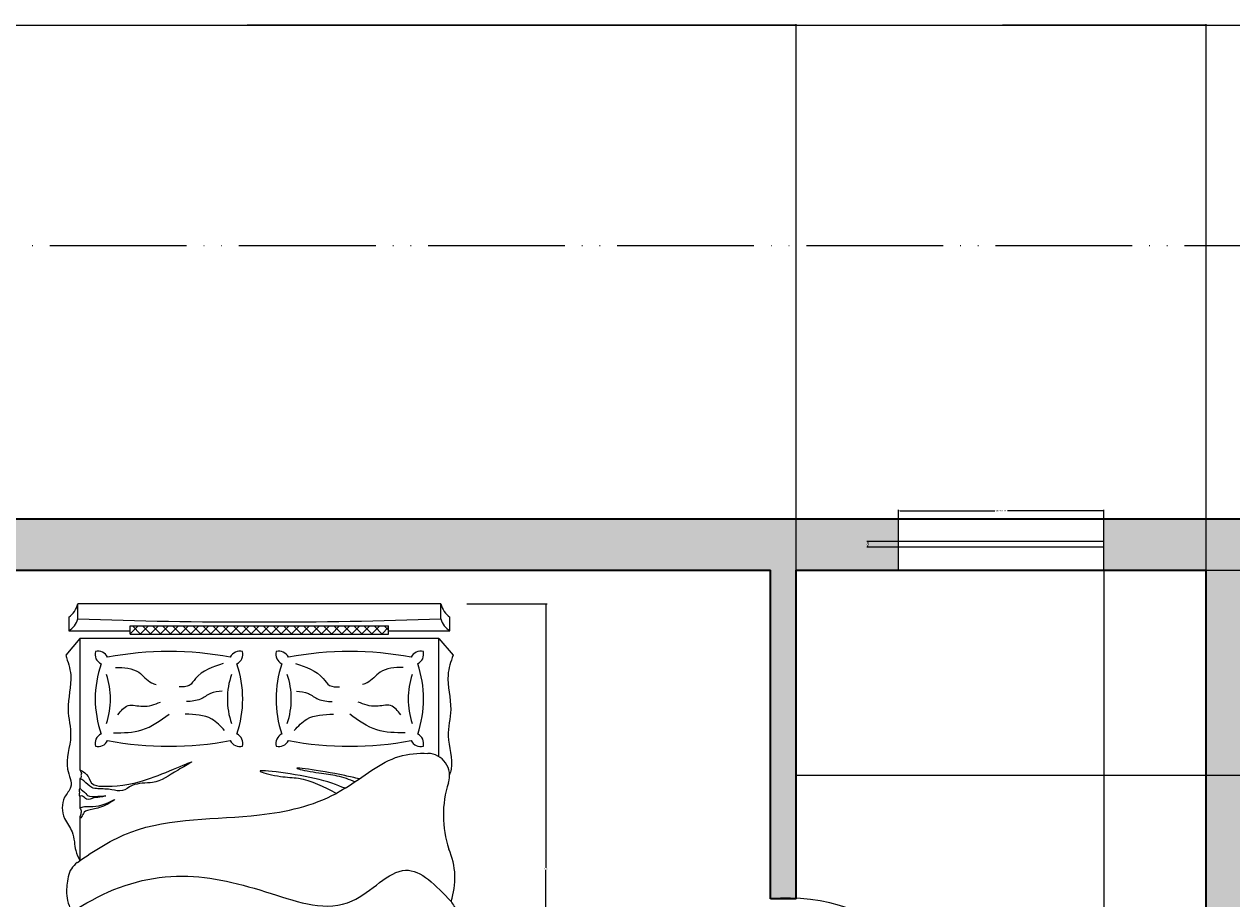
# Model space of a CAD drawing. Units: inches. Extents: x 2847 to 3693, y 1516 to 2098.
# Tile 4 of 6: x 3047 to 3259, y 1944 to 2098. Entities that reach past the tile are written whole.
import ezdxf

# ---------------------------------------------------------------- set-up
doc = ezdxf.new("R2010")
doc.units = ezdxf.units.IN
doc.linetypes.add('ACAD_ISO05W100', pattern=[33, 24, -3, 0, -3, 0, -3])
for name, color, linetype, lineweight in [('A-ANNO-DIMS', 2, 'Continuous', 18), ('A-DOOR', 3, 'Continuous', 18), ('A-FLOR-FIXT', 9, 'Continuous', 18), ('A-FURN', 8, 'Continuous', 18), ('A-GLAZ', 4, 'Continuous', 18), ('A-WALL', 7, 'Continuous', 35), ('C-PROP', 7, 'ACAD_ISO05W100', 18), ('www.cadblocksfree.com', 7, 'Continuous', 9)]:
    doc.layers.add(name, color=color, linetype=linetype, lineweight=lineweight)
doc.layers.add('A-WALL-PATT', color=251, linetype='Continuous', lineweight=13, true_color=0x636466)
doc.styles.get("Standard").update_dxf_attribs({"font": 'arial.ttf'})
doc.dimstyles.get("Standard").update_dxf_attribs({"dimtxt": 0.18, "dimasz": 0.18, "dimexe": 0.18, "dimexo": 0.0625, "dimgap": 0.09, "dimtad": 0, "dimtih": 1, "dimtoh": 1, "dimdec": 4, "dimzin": 0, "dimdsep": 46, "dimtxsty": 'Standard', "dimcen": 0.09, "dimadec": 0, "dimazin": 0, "dimtfac": 1, "dimtdec": 4, "dimtofl": 0, "dimtmove": 0, "dimatfit": 3, "dimfxl": 1, "dimtolj": 1, "dimtzin": 0, "dimarcsym": 0})

# ---------------------------------------------------------------- blocks, each defined once
blk = doc.blocks.new('bed')
at = {"layer": 'www.cadblocksfree.com', "ltscale": 0.2}
h = blk.add_hatch(dxfattribs=at)
h.set_pattern_fill('ANSI37,_O', color=256, scale=0.393701)
h.set_pattern_definition([(45, (2420.7222, -262.9689), (-0.8838835, 0.8838835), []), (135, (2420.7222, -262.9689), (-0.8838835, -0.8838835), [])])
h.paths.add_polyline_path([(3417.57, 1472.4), (3372.19, 1472.4), (3372.19, 1470.94), (3417.57, 1470.94)])
for p, q in [((3363, 1473.59), (3363, 1476.25)), ((3426.76, 1473.59), (3426.76, 1476.25)), ((3372.19, 1472.4), (3417.57, 1472.4)), ((3372.19, 1470.94), (3372.19, 1472.4)), ((3417.57, 1470.94), (3417.57, 1472.4)), ((3363.39, 1470.15), (3360.88, 1467.22)), ((3372.19, 1470.94), (3417.57, 1470.94)), ((3426.38, 1470.15), (3428.88, 1467.22)), ((3409.94, 1443.85), (3408.41, 1442.96)), ((3363.39, 1412.3), (3363.39, 1402.94)), ((3426.38, 1399.91), (3426.38, 1410.81)), ((3363.39, 1391.41), (3426.38, 1391.41))]:
    blk.add_line(p, q, dxfattribs=at)
for points in [[(3426.76, 1476.25), (3363, 1476.25)], [(3361.42, 1473.89), (3361.42, 1471.52), (3372.19, 1471.52)], [(3417.57, 1471.52), (3428.35, 1471.52), (3428.35, 1473.89)], [(3426.38, 1449.41), (3426.38, 1470.15), (3363.39, 1470.15), (3363.39, 1447.08)], [(3363.39, 1445.54), (3363.39, 1443.89)], [(3363.39, 1442.49), (3363.39, 1440.37)], [(3363.39, 1438.56), (3363.39, 1431.14)]]:
    blk.add_lwpolyline(points, dxfattribs=at)
for centre, radius, start, end in [((3359.33, 1477), 3.74, 303.8271, 348.4775), ((3430.43, 1477), 3.74, 191.5225, 236.1729), ((3359.84, 1474.37), 3.25, 298.9176, 345.9939), ((3394.88, 2431.36), 958.3, 268.09356, 271.90644), ((3429.92, 1474.37), 3.25, 194.0061, 241.0824), ((3367.9, 1467.4), 1.87, 165.5166, 244.2099), ((3366.56, 1466.05), 1.87, 25.7901, 104.4834), ((3379.01, 1409.19), 58.68, 79.4235, 100.5765), ((3391.47, 1466.05), 1.87, 75.5166, 154.2099), ((3390.12, 1467.4), 1.87, 295.7901, 14.4834), ((3399.64, 1467.4), 1.87, 165.5166, 244.2099), ((3398.3, 1466.05), 1.87, 25.7901, 104.4834), ((3410.75, 1409.19), 58.68, 79.4235, 100.5765), ((3423.21, 1466.05), 1.87, 75.5166, 154.2099), ((3421.86, 1467.4), 1.87, 295.7901, 14.4834), ((3385.29, 1459.55), 19.22, 161.2852, 198.7148), ((3372.74, 1459.55), 19.22, 341.2852, 18.7148), ((3417.03, 1459.55), 19.22, 161.2852, 198.7148), ((3404.48, 1459.55), 19.22, 341.2852, 18.7148), ((3355.42, 1459.55), 13.34, 341.1598, 18.8402), ((3402.61, 1459.55), 13.34, 161.1598, 198.8402), ((3387.15, 1459.55), 13.34, 341.1598, 18.8402), ((3434.35, 1459.55), 13.34, 161.1598, 198.8402), ((3367.9, 1451.7), 1.87, 115.7901, 194.4834), ((3390.12, 1451.7), 1.87, 345.5166, 64.2099), ((3399.64, 1451.7), 1.87, 115.7901, 194.4834), ((3421.86, 1451.7), 1.87, 345.5166, 64.2099), ((3366.56, 1453.04), 1.87, 255.5166, 334.2099), ((3379.01, 1509.91), 58.68, 259.4235, 280.5765), ((3391.47, 1453.04), 1.87, 205.7901, 284.4834), ((3398.3, 1453.04), 1.87, 255.5166, 334.2099), ((3410.75, 1509.91), 58.68, 259.4235, 280.5765), ((3423.21, 1453.04), 1.87, 205.7901, 284.4834), ((3424.34, 1446.05), 3.94, 342.0511, 87.9851), ((3445.78, 1439.1), 18.6, 162.0511, 198.5657), ((3416.57, 1428.08), 12.65, 341.0268, 23.7782), ((3365.21, 1427.6), 3.94, 125.4209, 169.6982), ((3370.55, 1414.19), 11.47, 139.4648, 203.3712), ((3367.28, 1412.87), 7.94, 204.0179, 212.619), ((3331.91, 1405.56), 34.38, 336.8495, 357.9003), ((3438.82, 1397.31), 13.77, 176.7525, 205.373), ((3432.14, 1393.64), 6.17, 162.6475, 201.1361), ((3422.11, 1384.8), 7.8, 58.0013, 91.6551)]:
    blk.add_arc(centre, radius, start, end, dxfattribs=at)
at = {"layer": 'www.cadblocksfree.com', "ltscale": 0.2, "extrusion": (0, 0, -1)}
for centre, major_axis, ratio, start_param, end_param in [((3360.34, 1388.37), (3.04, 3.04), 0.168252, 4.250342, 8.316029), ((3359.29, 1387.32), (1.05, 1.05), 0.453532, 4.422107, 8.144264)]:
    blk.add_ellipse(centre, major_axis=major_axis, ratio=ratio, start_param=start_param, end_param=end_param, dxfattribs=at)
at = {"layer": 'www.cadblocksfree.com', "ltscale": 0.2}
for centre, major_axis, ratio, start_param, end_param in [((3429.42, 1388.37), (-3.04, 3.04), 0.168252, 4.250342, 8.316029), ((3430.48, 1387.32), (-1.05, 1.05), 0.453532, 4.422107, 8.144264)]:
    blk.add_ellipse(centre, major_axis=major_axis, ratio=ratio, start_param=start_param, end_param=end_param, dxfattribs=at)
for points, knots in [([(3360.88, 1467.22), (3361.27, 1466.08), (3362.33, 1462.98), (3360.73, 1458.15), (3362.39, 1452.62), (3360.35, 1448.14), (3362.43, 1444.24), (3360.04, 1441.93), (3360.26, 1438.68), (3362.05, 1436.55), (3362.42, 1434.52), (3362.57, 1432.76), (3363.1, 1431.71), (3363.39, 1431.14)], [0, 0, 0, 0, 3.550403, 9.643115, 14.356056, 20.206026, 23.427697, 25.46537, 29.172767, 31.884544, 33.668442, 35.237641, 37.145618, 37.145618, 37.145618, 37.145618]), ([(3428.88, 1467.22), (3428.49, 1466.08), (3427.44, 1462.98), (3429.04, 1458.15), (3427.38, 1452.62), (3429.08, 1448.87), (3428.37, 1446.52), (3428.27, 1446.19)], [0, 0, 0, 0, 0.0901802, 0.2449351, 0.3646438, 0.5132331, 0.5378548, 0.5378548, 0.5378548, 0.5378548]), ([(3369.63, 1465.08), (3371.1, 1465.04), (3373.63, 1464.97), (3375.26, 1462.52), (3376.48, 1462.17), (3376.75, 1462.09)], [0, 0, 0, 0, 4.163459, 7.093919, 7.934624, 7.934624, 7.934624, 7.934624]), ([(3388.54, 1465.74), (3386.72, 1465.16), (3384.36, 1464.41), (3382.68, 1461.63), (3381.45, 1461.64), (3380.81, 1461.64)], [0, 0, 0, 0, 5.530688, 7.154877, 8.940839, 8.940839, 8.940839, 8.940839]), ([(3401.22, 1465.74), (3403.05, 1465.16), (3405.41, 1464.41), (3407.09, 1461.63), (3408.31, 1461.64), (3408.95, 1461.64)], [0, 0, 0, 0, 5.530688, 7.154877, 8.940839, 8.940839, 8.940839, 8.940839]), ([(3420.14, 1465.08), (3418.66, 1465.04), (3416.14, 1464.97), (3414.5, 1462.52), (3413.28, 1462.17), (3413.01, 1462.09)], [0, 0, 0, 0, 4.163459, 7.093919, 7.934624, 7.934624, 7.934624, 7.934624]), ([(3388.36, 1460.93), (3387.64, 1460.85), (3386.25, 1460.69), (3384.48, 1459.22), (3382.96, 1459.13), (3382.11, 1459.07)], [0, 0, 0, 0, 2.127543, 4.10272, 6.58647, 6.58647, 6.58647, 6.58647]), ([(3401.41, 1460.93), (3402.13, 1460.85), (3403.51, 1460.69), (3405.28, 1459.22), (3406.81, 1459.13), (3407.65, 1459.07)], [0, 0, 0, 0, 2.127543, 4.10272, 6.58647, 6.58647, 6.58647, 6.58647]), ([(3370.05, 1456.77), (3370.59, 1457.46), (3371.71, 1458.88), (3374.68, 1457.89), (3376.51, 1458.59), (3377.52, 1458.99)], [0, 0, 0, 0, 2.388143, 4.935423, 8.166198, 8.166198, 8.166198, 8.166198]), ([(3419.72, 1456.77), (3419.17, 1457.46), (3418.05, 1458.88), (3415.08, 1457.89), (3413.26, 1458.59), (3412.24, 1458.99)], [0, 0, 0, 0, 2.388143, 4.935423, 8.166198, 8.166198, 8.166198, 8.166198]), ([(3369.29, 1453.58), (3371, 1453.6), (3374.59, 1453.64), (3377.5, 1455.76), (3379.02, 1456.87)], [0, 0, 0, 0, 5.002087, 10.507046, 10.507046, 10.507046, 10.507046]), ([(3388.77, 1454), (3388.07, 1454.76), (3386.27, 1456.73), (3383.54, 1456.81), (3381.88, 1456.86)], [0, 0, 0, 0, 3.013696, 7.735839, 7.735839, 7.735839, 7.735839]), ([(3401, 1454), (3401.7, 1454.76), (3403.5, 1456.73), (3406.22, 1456.81), (3407.88, 1456.86)], [0, 0, 0, 0, 3.013696, 7.735839, 7.735839, 7.735839, 7.735839]), ([(3420.48, 1453.58), (3418.77, 1453.6), (3415.18, 1453.64), (3412.27, 1455.76), (3410.74, 1456.87)], [0, 0, 0, 0, 5.002087, 10.507046, 10.507046, 10.507046, 10.507046]), ([(3367.27, 1444.2), (3369.57, 1444.23), (3373.92, 1444.28), (3385.47, 1449.8), (3379.56, 1446.49), (3376.81, 1444.48), (3372.95, 1444.92), (3370.93, 1443.14), (3368.77, 1443.7), (3367.36, 1443.75), (3366.55, 1443.78)], [0, 0, 0, 0, 8.61026, 16.221274, 18.843057, 23.804898, 27.440828, 29.356102, 31.203478, 33.650687, 33.650687, 33.650687, 33.650687]), ([(3409.94, 1443.85), (3413.12, 1445.84), (3417.43, 1449.66), (3422.72, 1450.04), (3424.48, 1449.98)], [1.3582378, 1.3582378, 1.3582378, 1.3582378, 1.6381418, 1.7706953, 1.7706953, 1.7706953, 1.7706953]), ([(3363.39, 1447.08), (3363.43, 1446.99), (3363.53, 1446.78), (3363.73, 1446.46), (3363.51, 1446.15), (3363.66, 1445.9), (3363.56, 1445.67), (3363.44, 1445.58), (3363.39, 1445.54)], [0, 0, 0, 0, 0.293454, 0.701471, 1.003873, 1.254893, 1.47342, 1.69185, 1.69185, 1.69185, 1.69185]), ([(3363.39, 1447.08), (3363.99, 1446.78), (3365.08, 1446.12), (3365.12, 1444.37), (3367.13, 1444.19), (3367.27, 1444.2)], [0.0122268, 0.0122268, 0.0122268, 0.0122268, 0.0594721, 0.1062177, 0.134458, 0.134458, 0.134458, 0.134458]), ([(3409.94, 1443.85), (3408.47, 1444.45), (3404.44, 1446.04), (3391.4, 1447.6), (3398.64, 1445.77), (3402.97, 1445.76), (3406.22, 1444.09), (3408.41, 1442.96)], [0.0056315, 0.0056315, 0.0056315, 0.0056315, 0.1489731, 0.3882761, 0.4793617, 0.5593494, 0.7397317, 0.7397317, 0.7397317, 0.7397317]), ([(3412.4, 1445.5), (3411.61, 1445.7), (3406.24, 1446.93), (3398.17, 1447.93), (3405.4, 1446.46), (3408.57, 1446.19), (3410.63, 1445.46), (3411.68, 1445)], [0.1043639, 0.1043639, 0.1043639, 0.1043639, 0.1489731, 0.3882761, 0.4793617, 0.5593494, 0.6446217, 0.6446217, 0.6446217, 0.6446217]), ([(3363.39, 1443.89), (3363.33, 1443.81), (3363.17, 1443.56), (3363.35, 1443.12), (3363.23, 1442.79), (3363.23, 1442.53), (3363.34, 1442.51), (3363.39, 1442.49)], [0, 0, 0, 0, 0.27176, 0.887321, 1.189132, 1.388142, 1.515331, 1.515331, 1.515331, 1.515331]), ([(3366.55, 1443.78), (3366.17, 1443.78), (3365.17, 1443.9), (3364.4, 1444.96), (3363.63, 1445.46), (3363.39, 1445.54)], [0.15648839, 0.15648839, 0.15648839, 0.15648839, 0.18439755, 0.23137648, 0.25059846, 0.25059846, 0.25059846, 0.25059846]), ([(3363.39, 1443.89), (3363.63, 1443.61), (3364.67, 1442.73), (3364.89, 1442.15), (3369.07, 1442.74), (3366.77, 1442.24), (3365.83, 1442.3), (3364.61, 1441.55), (3363.96, 1442.54), (3363.54, 1442.52), (3363.39, 1442.49)], [0.0595743, 0.0595743, 0.0595743, 0.0595743, 0.0807529, 0.1037415, 0.1697201, 0.1760361, 0.2071372, 0.2404744, 0.2623409, 0.2736605, 0.2736605, 0.2736605, 0.2736605]), ([(3362.93, 1430.81), (3365.94, 1432.96), (3375.45, 1438.99), (3392.12, 1438.03), (3404.25, 1440.73), (3408.41, 1442.96)], [0.102872, 0.102872, 0.102872, 0.102872, 0.37972, 0.957702, 1.313793, 1.313793, 1.313793, 1.313793]), ([(3363.39, 1440.37), (3363.63, 1440.51), (3364.53, 1440.9), (3366.48, 1440.25), (3370.2, 1442.29), (3367.73, 1440.64), (3365.42, 1440.07), (3364.04, 1439.91), (3363.8, 1438.94), (3363.48, 1438.64), (3363.39, 1438.56)], [0.013856, 0.013856, 0.013856, 0.013856, 0.0348738, 0.0888667, 0.1078792, 0.1267378, 0.158714, 0.1937575, 0.2174868, 0.2267221, 0.2267221, 0.2267221, 0.2267221]), ([(3363.39, 1440.37), (3363.44, 1440.27), (3363.57, 1440.06), (3363.61, 1439.68), (3363.53, 1439.31), (3363.41, 1439), (3363.33, 1438.75), (3363.37, 1438.61), (3363.39, 1438.56)], [0, 0, 0, 0, 0.329977, 0.725302, 1.129072, 1.442831, 1.734218, 1.878348, 1.878348, 1.878348, 1.878348]), ([(3365.51, 1424.21), (3370.52, 1427), (3381.15, 1429.83), (3396.21, 1425.87), (3410.54, 1420.65), (3420.27, 1432.69), (3425.88, 1426.77), (3428.53, 1423.97)], [0.099185, 0.099185, 0.099185, 0.099185, 0.523647, 0.927087, 1.289918, 1.564439, 1.810555, 1.810555, 1.810555, 1.810555]), ([(3361.34, 1428.31), (3361.33, 1428.3), (3361.16, 1427.34), (3360.78, 1425.17), (3361.47, 1423.14), (3362.01, 1421.85)], [0.3128349, 0.3128349, 0.3128349, 0.3128349, 0.313751, 0.386958, 0.4759027, 0.4759027, 0.4759027, 0.4759027]), ([(3428.53, 1423.97), (3428.91, 1423.4), (3430.1, 1421.61), (3428.49, 1417.66), (3430.59, 1413.79), (3429.8, 1409.12), (3428.4, 1406.56), (3427.36, 1404.97)], [0, 0, 0, 0, 0.050513, 0.157399, 0.2842023, 0.3628173, 0.5066917, 0.5066917, 0.5066917, 0.5066917]), ([(3362.06, 1409.87), (3363.64, 1413.65), (3372.98, 1421.34), (3389.68, 1406.04), (3402.4, 1419.98), (3416.04, 1420.17), (3423.23, 1415.23), (3427.83, 1408.9)], [0.029901, 0.029901, 0.029901, 0.029901, 0.276967, 0.797115, 1.093669, 1.464666, 1.788489, 1.788489, 1.788489, 1.788489]), ([(3431.24, 1387.47), (3430.88, 1388.17), (3430.2, 1389.5), (3431.48, 1391.99), (3428.29, 1393.19), (3430.5, 1395.69), (3427.56, 1397.87), (3431.84, 1400.39), (3426.54, 1404.33), (3426.44, 1408.15), (3426.38, 1410.81)], [0, 0, 0, 0, 2.267059, 4.324559, 6.685584, 8.878641, 11.121502, 14.300359, 17.755284, 25.682856, 25.682856, 25.682856, 25.682856]), ([(3358.53, 1387.47), (3359.1, 1389.21), (3359.96, 1391.82), (3361.92, 1395.15), (3361.9, 1398.55), (3359.88, 1401.84), (3361.56, 1405.21), (3361.03, 1407.51), (3360.64, 1408.47), (3360.59, 1408.59)], [0, 0, 0, 0, 0.138875, 0.2092702, 0.2901949, 0.3858479, 0.4804923, 0.5489252, 0.5590752, 0.5590752, 0.5590752, 0.5590752]), ([(3368.63, 1397.84), (3375.98, 1400.49), (3385.35, 1402.76), (3397.53, 1395.27), (3413.59, 1410.38), (3407.81, 1395.02), (3420.76, 1398.2)], [0.029901, 0.029901, 0.029901, 0.029901, 0.276967, 0.797115, 1.093669, 1.16836, 1.16836, 1.16836, 1.16836]), ([(3430.32, 1386.56), (3427.33, 1387.65), (3422.15, 1389.55), (3414.53, 1384.14), (3405.61, 1387.05), (3396.29, 1386.31), (3386.84, 1381.28), (3377.74, 1390.27), (3370.78, 1384.8), (3364.63, 1383.97), (3363.28, 1388.27), (3360.78, 1387.15), (3359.45, 1386.56)], [0, 0, 0, 0, 8.93042, 15.449194, 25.485629, 34.878505, 43.598887, 54.554403, 64.16647, 67.461673, 70.610457, 74.213583, 74.213583, 74.213583, 74.213583])]:
    blk.add_open_spline(points, degree=3, knots=knots, dxfattribs=at)
for points in [[(3361.23, 1424.04), (3361.24, 1424.04), (3361.24, 1424.04), (3361.24, 1424.04)], [(3361.84, 1421.64), (3362.35, 1422.25), (3362.87, 1422.86), (3365.51, 1424.21)]]:
    blk.add_open_spline(points, degree=3, dxfattribs=at)
blk = doc.blocks.new('WIN-GLAZ-36IN')
for p, q in [((36, 1), (0, 1)), ((36, 0), (0, 0))]:
    blk.add_line(p, q)
blk = doc.blocks.new('*D17')
at = {"layer": 'A-ANNO-DIMS', "color": 0, "lineweight": -2, "transparency": 16777216}
for p, q in [((3200.85, 2007.18), (3200.85, 2012.7)), ((3201.03, 2012.52), (3217.73, 2012.52)), ((3236.67, 2012.52), (3219.96, 2012.52)), ((3236.85, 2007.18), (3236.85, 2012.7))]:
    blk.add_line(p, q, dxfattribs=at)
at = {"layer": 'A-ANNO-DIMS', "color": 0, "transparency": 16777216}
for points in [[(3201.03, 2012.55), (3201.03, 2012.49), (3200.85, 2012.52)], [(3236.67, 2012.55), (3236.67, 2012.49), (3236.85, 2012.52)]]:
    blk.add_solid(points, dxfattribs=at)
at = {"layer": 'Defpoints', "color": 0, "transparency": 16777216}
for p in [(3236.85, 2012.52), (3200.85, 2007.12), (3236.85, 2007.12)]:
    blk.add_point(p, dxfattribs=at)
at = {"layer": 'A-ANNO-DIMS', "color": 0, "transparency": 16777216, "insert": (3218.85, 2012.52), "char_height": 0.18, "attachment_point": 5}
blk.add_mtext('\\A1;WINDOW 36 TYP.', dxfattribs=at)
blk = doc.blocks.new('*D18')
at = {"layer": 'A-ANNO-DIMS', "color": 0, "lineweight": -2, "transparency": 16777216}
for p, q in [((3200.78, 2007.12), (3195.27, 2007.12)), ((3200.78, 2006.12), (3195.27, 2006.12)), ((3195.45, 2006.94), (3195.45, 2006.8)), ((3195.45, 2006.3), (3195.45, 2006.44))]:
    blk.add_line(p, q, dxfattribs=at)
at = {"layer": 'A-ANNO-DIMS', "color": 0, "transparency": 16777216}
for points in [[(3195.42, 2006.94), (3195.48, 2006.94), (3195.45, 2007.12)], [(3195.42, 2006.3), (3195.48, 2006.3), (3195.45, 2006.12)]]:
    blk.add_solid(points, dxfattribs=at)
at = {"layer": 'Defpoints', "color": 0, "transparency": 16777216}
for p in [(3195.45, 2007.12), (3200.85, 2007.12), (3200.85, 2006.12)]:
    blk.add_point(p, dxfattribs=at)
at = {"layer": 'A-ANNO-DIMS', "color": 0, "transparency": 16777216, "insert": (3195.45, 2006.62), "char_height": 0.18, "attachment_point": 5}
blk.add_mtext('\\A1;1 TYP.', dxfattribs=at)
blk = doc.blocks.new('*D21')
at = {"layer": 'A-ANNO-DIMS', "color": 0, "lineweight": -2, "transparency": 16777216}
for p, q in [((3125.04, 1996.19), (3139.12, 1996.19)), ((3138.94, 1996.01), (3138.94, 1949.83)), ((3138.94, 1903.3), (3138.94, 1949.47)), ((3125.04, 1903.12), (3139.12, 1903.12))]:
    blk.add_line(p, q, dxfattribs=at)
at = {"layer": 'A-ANNO-DIMS', "color": 0, "transparency": 16777216}
for points in [[(3138.91, 1996.01), (3138.97, 1996.01), (3138.94, 1996.19)], [(3138.91, 1903.3), (3138.97, 1903.3), (3138.94, 1903.12)]]:
    blk.add_solid(points, dxfattribs=at)
at = {"layer": 'Defpoints', "color": 0, "transparency": 16777216}
for p in [(3124.97, 1996.19), (3138.94, 1996.19), (3124.97, 1903.12)]:
    blk.add_point(p, dxfattribs=at)
at = {"layer": 'A-ANNO-DIMS', "color": 0, "transparency": 16777216, "insert": (3138.94, 1949.65), "char_height": 0.18, "attachment_point": 5}
blk.add_mtext('\\A1;BED 93', dxfattribs=at)
blk = doc.blocks.new('*D35')
at = {"layer": 'A-ANNO-DIMS', "color": 0, "lineweight": -2, "transparency": 16777216}
for p, q in [((2885.85, 2059.18), (2885.85, 2098)), ((2886.03, 2097.82), (3269.56, 2097.82)), ((3653.67, 2097.82), (3270.13, 2097.82)), ((3653.85, 2059.18), (3653.85, 2098))]:
    blk.add_line(p, q, dxfattribs=at)
at = {"layer": 'A-ANNO-DIMS', "color": 0, "transparency": 16777216}
for points in [[(2886.03, 2097.85), (2886.03, 2097.79), (2885.85, 2097.82)], [(3653.67, 2097.85), (3653.67, 2097.79), (3653.85, 2097.82)]]:
    blk.add_solid(points, dxfattribs=at)
at = {"layer": 'Defpoints', "color": 0, "transparency": 16777216}
for p in [(3653.85, 2097.82), (2885.85, 2059.12), (3653.85, 2059.12)]:
    blk.add_point(p, dxfattribs=at)
at = {"layer": 'A-ANNO-DIMS', "color": 0, "transparency": 16777216, "insert": (3269.85, 2097.82), "char_height": 0.18, "attachment_point": 5}
blk.add_mtext('\\A1;768', dxfattribs=at)
blk = doc.blocks.new('*D39')
at = {"layer": 'A-ANNO-DIMS', "color": 0, "lineweight": -2, "transparency": 16777216}
for p, q in [((2989.35, 2011.18), (2989.35, 2098)), ((2989.53, 2097.82), (3085.71, 2097.82)), ((3182.67, 2097.82), (3086.48, 2097.82)), ((3182.85, 2002.18), (3182.85, 2098))]:
    blk.add_line(p, q, dxfattribs=at)
at = {"layer": 'A-ANNO-DIMS', "color": 0, "transparency": 16777216}
for points in [[(2989.53, 2097.85), (2989.53, 2097.79), (2989.35, 2097.82)], [(3182.67, 2097.85), (3182.67, 2097.79), (3182.85, 2097.82)]]:
    blk.add_solid(points, dxfattribs=at)
at = {"layer": 'Defpoints', "color": 0, "transparency": 16777216}
for p in [(3182.85, 2097.82), (2989.35, 2011.12), (3182.85, 2002.12)]:
    blk.add_point(p, dxfattribs=at)
at = {"layer": 'A-ANNO-DIMS', "color": 0, "transparency": 16777216, "insert": (3086.1, 2097.82), "char_height": 0.18, "attachment_point": 5}
blk.add_mtext('\\A1;193.5', dxfattribs=at)
blk = doc.blocks.new('*D40')
at = {"layer": 'A-ANNO-DIMS', "color": 0, "lineweight": -2, "transparency": 16777216}
for p, q in [((3182.85, 2002.18), (3182.85, 2098)), ((3183.03, 2097.82), (3218.63, 2097.82)), ((3254.67, 2097.82), (3219.06, 2097.82)), ((3254.85, 2002.18), (3254.85, 2098))]:
    blk.add_line(p, q, dxfattribs=at)
at = {"layer": 'A-ANNO-DIMS', "color": 0, "transparency": 16777216}
for points in [[(3183.03, 2097.85), (3183.03, 2097.79), (3182.85, 2097.82)], [(3254.67, 2097.85), (3254.67, 2097.79), (3254.85, 2097.82)]]:
    blk.add_solid(points, dxfattribs=at)
at = {"layer": 'Defpoints', "color": 0, "transparency": 16777216}
for p in [(3254.85, 2097.82), (3182.85, 2002.12), (3254.85, 2002.12)]:
    blk.add_point(p, dxfattribs=at)
at = {"layer": 'A-ANNO-DIMS', "color": 0, "transparency": 16777216, "insert": (3218.85, 2097.82), "char_height": 0.18, "attachment_point": 5}
blk.add_mtext('\\A1;72', dxfattribs=at)
blk = doc.blocks.new('*D41')
at = {"layer": 'A-ANNO-DIMS', "color": 0, "lineweight": -2, "transparency": 16777216}
for p, q in [((3254.85, 2002.18), (3254.85, 2098)), ((3255.03, 2097.82), (3337.06, 2097.82)), ((3419.67, 2097.82), (3337.63, 2097.82)), ((3419.85, 2002.18), (3419.85, 2098))]:
    blk.add_line(p, q, dxfattribs=at)
at = {"layer": 'A-ANNO-DIMS', "color": 0, "transparency": 16777216}
for points in [[(3255.03, 2097.85), (3255.03, 2097.79), (3254.85, 2097.82)], [(3419.67, 2097.85), (3419.67, 2097.79), (3419.85, 2097.82)]]:
    blk.add_solid(points, dxfattribs=at)
at = {"layer": 'Defpoints', "color": 0, "transparency": 16777216}
for p in [(3419.85, 2097.82), (3254.85, 2002.12), (3419.85, 2002.12)]:
    blk.add_point(p, dxfattribs=at)
at = {"layer": 'A-ANNO-DIMS', "color": 0, "transparency": 16777216, "insert": (3337.35, 2097.82), "char_height": 0.18, "attachment_point": 5}
blk.add_mtext('\\A1;165', dxfattribs=at)
blk = doc.blocks.new('*D50')
at = {"layer": 'A-ANNO-DIMS', "color": 0, "lineweight": -2, "transparency": 16777216}
for p, q in [((2989.41, 2011.12), (3692.73, 2011.12)), ((3692.55, 2010.94), (3692.55, 1924.3)), ((3692.55, 1837.3), (3692.55, 1923.94)), ((2989.41, 1837.12), (3692.73, 1837.12))]:
    blk.add_line(p, q, dxfattribs=at)
at = {"layer": 'A-ANNO-DIMS', "color": 0, "transparency": 16777216}
for points in [[(3692.52, 2010.94), (3692.58, 2010.94), (3692.55, 2011.12)], [(3692.52, 1837.3), (3692.58, 1837.3), (3692.55, 1837.12)]]:
    blk.add_solid(points, dxfattribs=at)
at = {"layer": 'Defpoints', "color": 0, "transparency": 16777216}
for p in [(2989.35, 2011.12), (3692.55, 2011.12), (2989.35, 1837.12)]:
    blk.add_point(p, dxfattribs=at)
at = {"layer": 'A-ANNO-DIMS', "color": 0, "transparency": 16777216, "insert": (3692.55, 1924.12), "char_height": 0.18, "attachment_point": 5}
blk.add_mtext('\\A1;174', dxfattribs=at)
blk = doc.blocks.new('*D75')
at = {"layer": 'A-ANNO-DIMS', "color": 0, "lineweight": -2, "transparency": 16777216}
for p, q in [((3236.85, 2002.06), (3236.85, 1516.24)), ((3254.85, 2002.06), (3254.85, 1516.24)), ((3237.03, 1516.42), (3245.64, 1516.42)), ((3254.67, 1516.42), (3246.06, 1516.42))]:
    blk.add_line(p, q, dxfattribs=at)
at = {"layer": 'A-ANNO-DIMS', "color": 0, "transparency": 16777216}
for points in [[(3237.03, 1516.45), (3237.03, 1516.39), (3236.85, 1516.42)], [(3254.67, 1516.45), (3254.67, 1516.39), (3254.85, 1516.42)]]:
    blk.add_solid(points, dxfattribs=at)
at = {"layer": 'Defpoints', "color": 0, "transparency": 16777216}
for p in [(3236.85, 2002.12), (3254.85, 2002.12), (3254.85, 1516.42)]:
    blk.add_point(p, dxfattribs=at)
at = {"layer": 'A-ANNO-DIMS', "color": 0, "transparency": 16777216, "insert": (3245.85, 1516.42), "char_height": 0.18, "attachment_point": 5}
blk.add_mtext('\\A1;18', dxfattribs=at)
blk = doc.blocks.new('*D79')
at = {"layer": 'A-ANNO-DIMS', "color": 0, "lineweight": -2, "transparency": 16777216}
for p, q in [((3182.91, 2002.12), (3692.73, 2002.12)), ((3692.55, 2001.94), (3692.55, 1984.3)), ((3692.55, 1966.3), (3692.55, 1983.94)), ((3182.91, 1966.12), (3692.73, 1966.12))]:
    blk.add_line(p, q, dxfattribs=at)
at = {"layer": 'A-ANNO-DIMS', "color": 0, "transparency": 16777216}
for points in [[(3692.52, 2001.94), (3692.58, 2001.94), (3692.55, 2002.12)], [(3692.52, 1966.3), (3692.58, 1966.3), (3692.55, 1966.12)]]:
    blk.add_solid(points, dxfattribs=at)
at = {"layer": 'Defpoints', "color": 0, "transparency": 16777216}
for p in [(3182.85, 2002.12), (3692.55, 2002.12), (3182.85, 1966.12)]:
    blk.add_point(p, dxfattribs=at)
at = {"layer": 'A-ANNO-DIMS', "color": 0, "transparency": 16777216, "insert": (3692.55, 1984.12), "char_height": 0.18, "attachment_point": 5}
blk.add_mtext('\\A1;36', dxfattribs=at)

msp = doc.modelspace()

# ---------------------------------------------------------------- hatches: boundary and pattern name
at = {"layer": 'A-WALL-PATT'}
h = msp.add_hatch(color=256, dxfattribs=at)
h.dxf.hatch_style = 1
h.paths.add_polyline_path([(2998.3457, 2002.118), (3178.3457, 2002.118), (3178.3457, 1944.368, -0.0341147), (3182.8457, 1944.4698), (3182.8457, 2002.118), (3200.8457, 2002.118), (3200.8457, 2011.118), (2989.3457, 2011.118), (2989.3457, 1960.118), (2998.3457, 1960.118)])
h.paths.add_polyline_path([(2998.3457, 1888.118), (2989.3457, 1888.118), (2989.3457, 1837.118), (3089.8457, 1837.118), (3089.8457, 1778.618), (3098.8457, 1778.618), (3098.8457, 1837.118), (3130.3457, 1837.118, -0.05293254), (3130.1282, 1846.118), (2998.3457, 1846.118)])
h.paths.add_polyline_path([(3263.8457, 2002.118), (3311.8457, 2002.118), (3311.8457, 2011.118), (3263.8457, 2011.118), (3236.8457, 2011.118), (3236.8457, 2002.118), (3254.8457, 2002.118), (3254.8457, 1908.368), (3182.8457, 1908.368), (3178.3457, 1908.368), (3178.3457, 1886.993), (3182.8457, 1886.993), (3182.8457, 1903.868), (3254.8457, 1903.868), (3254.8457, 1846.118), (3182.8457, 1846.118), (3182.8457, 1850.993), (3178.3457, 1850.993), (3178.3457, 1837.118), (3254.8457, 1837.118), (3254.8457, 1790.618), (3263.8457, 1790.618), (3263.8457, 1837.118)])
h.paths.add_polyline_path([(2930.8457, 1837.118), (2921.8457, 1837.118), (2921.8457, 1828.118), (2930.8457, 1828.118)])
h.paths.add_polyline_path([(2930.8457, 1600.118), (2921.8457, 1600.118), (2921.8457, 1591.118), (2930.8457, 1591.118)])
h.paths.add_polyline_path([(3098.8457, 1658.618), (3089.8457, 1658.618), (3089.8457, 1591.118), (3140.8457, 1591.118), (3140.8457, 1600.118), (3098.8457, 1600.118)])
h.paths.add_polyline_path([(3305.8457, 1600.118), (3263.8457, 1600.118), (3263.8457, 1646.618), (3254.8457, 1646.618), (3254.8457, 1600.118), (3212.8457, 1600.118), (3212.8457, 1591.118), (3254.8457, 1591.118), (3305.8457, 1591.118)])
h.paths.add_polyline_path([(3470.8457, 1600.118), (3428.8457, 1600.118), (3428.8457, 1756.118), (3430.26, 1756.118), (3430.26, 1765.118), (3428.8457, 1765.118), (3419.8457, 1765.118), (3419.8457, 1600.118), (3377.8457, 1600.118), (3377.8457, 1591.118), (3470.8457, 1591.118)])
h.paths.add_polyline_path([(3593.8457, 1642.118), (3584.8457, 1642.118), (3584.8457, 1600.118), (3542.8457, 1600.118), (3542.8457, 1591.118), (3593.8457, 1591.118)])
h.paths.add_polyline_path([(3593.8457, 1796.083), (3584.8457, 1796.083), (3584.8457, 1765.118), (3505.3457, 1765.118), (3505.3457, 1837.118), (3584.8457, 1837.118), (3584.8457, 1832.083), (3593.8457, 1832.083), (3593.8457, 1837.118), (3593.8457, 1924.118), (3584.8457, 1924.118), (3584.8457, 1846.118), (3478.26, 1846.118), (3478.26, 1837.118), (3500.8457, 1837.118), (3500.8457, 1765.118), (3478.26, 1765.118, -0.03536449), (3478.26, 1758.7816), (3478.26, 1756.118), (3584.8457, 1756.118), (3584.8457, 1714.118), (3593.8457, 1714.118)])
h.paths.add_polyline_path([(3593.8457, 2011.118), (3536.8457, 2011.118), (3536.8457, 2002.118), (3584.8457, 2002.118), (3584.8457, 1960.118), (3593.8457, 1960.118)])
h.paths.add_polyline_path([(3476.8457, 2011.118), (3371.8457, 2011.118), (3371.8457, 2002.118), (3419.8457, 2002.118), (3419.8457, 1837.118), (3428.8457, 1837.118), (3430.26, 1837.118), (3430.26, 1846.118), (3428.8457, 1846.118), (3428.8457, 2002.118), (3476.8457, 2002.118)])

# ---------------------------------------------------------------- linework, layer by layer
at = {"layer": 'A-DOOR'}
msp.add_arc((3181.3406, 1911.4803), 33.0238, 358.069858, 95.203296, dxfattribs=at)
at = {"layer": 'A-FLOR-FIXT'}
msp.add_line((3182.8457, 1966.118), (3254.8457, 1966.118), dxfattribs=at)
at = {"layer": 'A-GLAZ'}
for p, q in [((3200.8457, 2002.118), (3200.8457, 2011.118)), ((3236.8457, 2002.118), (3236.8457, 2011.118))]:
    msp.add_line(p, q, dxfattribs=at)
at = {"layer": 'A-WALL'}
for p, q in [((2989.3457, 2011.118), (3263.8457, 2011.118)), ((2998.3457, 2002.118), (3178.3457, 2002.118)), ((3178.3457, 1944.368), (3178.3457, 2002.118)), ((3182.8457, 2002.118), (3254.8457, 2002.118)), ((3182.8457, 1944.368), (3182.8457, 2002.118)), ((3254.8457, 1908.368), (3254.8457, 2002.118)), ((3182.8457, 1944.368), (3178.3457, 1944.368))]:
    msp.add_line(p, q, dxfattribs=at)
at = {"layer": 'C-PROP'}
msp.add_line((2885.8457, 2059.118), (3653.8457, 2059.118), dxfattribs=at)

# ---------------------------------------------------------------- block references
at = {"layer": 'A-FURN'}
msp.add_blockref('bed', (-306.2617, 519.939), dxfattribs=at)
at = {"layer": 'A-GLAZ'}
msp.add_blockref('WIN-GLAZ-36IN', (3200.846, 2006.118), dxfattribs=at)

# ---------------------------------------------------------------- dimensions: what is measured, and where the dimension line sits
at = {"layer": 'A-ANNO-DIMS'}
for base, p1, p2, override, picture, middle in [((3653.8457, 2097.818), (2885.8457, 2059.118), (3653.8457, 2059.118), {"dimdec": 0, "dimlfac": 1, "dimrnd": 0, "dimzin": 0, "dimdsep": 46, "dimlunit": 2}, '*D35', (3269.8457, 2097.818)), ((3182.8457, 2097.818), (2989.3457, 2011.118), (3182.8457, 2002.118), {"dimdec": 1, "dimlfac": 1, "dimrnd": 0, "dimzin": 0, "dimdsep": 46, "dimlunit": 2}, '*D39', (3086.0957, 2097.818)), ((3254.8457, 2097.818), (3182.8457, 2002.118), (3254.8457, 2002.118), {"dimdec": 0, "dimlfac": 1, "dimrnd": 0, "dimzin": 0, "dimdsep": 46, "dimlunit": 2}, '*D40', (3218.8457, 2097.818)), ((3419.8457, 2097.818), (3254.8457, 2002.118), (3419.8457, 2002.118), {"dimdec": 0, "dimlfac": 1, "dimrnd": 0, "dimzin": 0, "dimdsep": 46, "dimlunit": 2}, '*D41', (3337.3457, 2097.818)), ((3254.8457, 1516.418), (3236.8457, 2002.118), (3254.8457, 2002.118), {"dimdec": 0, "dimlfac": 1, "dimrnd": 0, "dimzin": 0, "dimdsep": 46, "dimlunit": 2}, '*D75', (3245.8457, 1516.418))]:
    dim = msp.add_linear_dim(base=base, p1=p1, p2=p2, dimstyle='Standard', override=override, dxfattribs=at)
    dim.commit()
    dim.dimension.update_dxf_attribs({"geometry": picture, "text_midpoint": middle})
dim = msp.add_linear_dim(base=(3236.8457, 2012.518), p1=(3200.8457, 2007.118), p2=(3236.8457, 2007.118), text='WINDOW <> TYP.', dimstyle='Standard', override={"dimdec": 0, "dimlfac": 1, "dimrnd": 0, "dimzin": 0, "dimdsep": 46, "dimlunit": 2}, dxfattribs=at)
dim.commit()
dim.dimension.update_dxf_attribs({"geometry": '*D17', "text_midpoint": (3218.8457, 2012.518)})
for base, p1, p2, picture, middle in [((3692.5457, 2011.118), (2989.3457, 1837.118), (2989.3457, 2011.118), '*D50', (3692.5457, 1924.118)), ((3692.5457, 2002.118), (3182.8457, 1966.118), (3182.8457, 2002.118), '*D79', (3692.5457, 1984.118))]:
    dim = msp.add_linear_dim(base=base, p1=p1, p2=p2, angle=90, dimstyle='Standard', override={"dimdec": 0, "dimlfac": 1, "dimrnd": 0, "dimzin": 0, "dimdsep": 46, "dimlunit": 2}, dxfattribs=at)
    dim.commit()
    dim.dimension.update_dxf_attribs({"geometry": picture, "text_midpoint": middle})
for base, p1, p2, text, picture, middle in [((3195.4457, 2007.118), (3200.8457, 2006.118), (3200.8457, 2007.118), '<> TYP.', '*D18', (3195.4457, 2006.618)), ((3138.9356, 1996.1877), (3124.975, 1903.1171), (3124.975, 1996.1877), 'BED <>', '*D21', (3138.9356, 1949.6524))]:
    dim = msp.add_linear_dim(base=base, p1=p1, p2=p2, angle=90, text=text, dimstyle='Standard', override={"dimdec": 0, "dimlfac": 1, "dimrnd": 0, "dimzin": 0, "dimdsep": 46, "dimlunit": 2}, dxfattribs=at)
    dim.commit()
    dim.dimension.update_dxf_attribs({"geometry": picture, "text_midpoint": middle})

doc.saveas('drawing.dxf')
